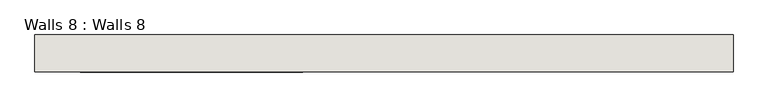
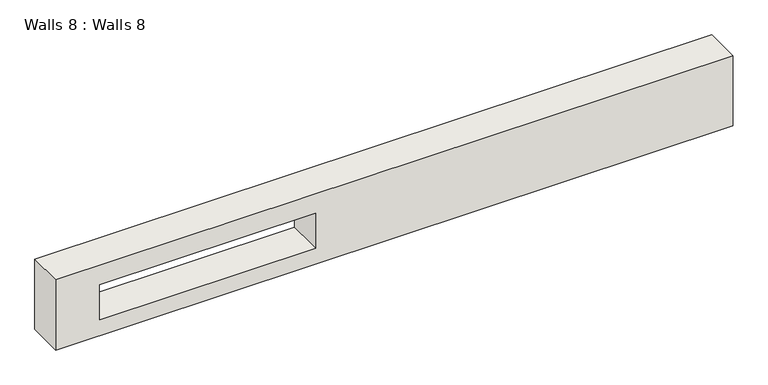
"""IFC4 building model written with IfcOpenShell, lengths in millimetres: wall geometry, Walls 8 : Walls 8."""

from ifc_helpers import new_model, si_unit, frame, origin, place, context, project, spatial, polyline, outline, extrude, source, transform, mapped, element, save


def walls_8_walls_8_f603c033(model_context):
    return source(origin(), model_context, "Body", "SweptSolid", [
        extrude(outline(polyline([(3969.8902454, 645.5980639), (3969.8902454, -5093.2019361), (3341.3717218, -5093.2019361), (3341.3717218, 645.5980639), (3969.8902454, 645.5980639)]), holes=[polyline([(3794.6218444, -2890.5343531), (3483.6009608, -2890.5343531), (3483.6009608, -4719.3343531), (3794.6218444, -4719.3343531), (3794.6218444, -2890.5343531)])]), frame((0.0, -6810.6562913, 0.0), z_axis=(0.0, 1.0, 0.0), x_axis=(0.0, 0.0, 1.0)), (0.0, 0.0, 1.0), 304.8),
    ])


if __name__ == "__main__":
    model = new_model("IFC4")
    model_context = context("Model", 3, world=origin())
    ifc_project = project(units=[si_unit("LENGTHUNIT", "METRE", prefix="MILLI")], contexts=[model_context])
    site = spatial("IfcSite", under=ifc_project)
    building = spatial("IfcBuilding", under=site)
    placement = place(None, origin())
    walls_8_walls_8_shape = walls_8_walls_8_f603c033(model_context)
    element("IfcWall", 1, ObjectType="Walls 8 : Walls 8", at=placement, inside=building, context=model_context, shape_type="MappedRepresentation", body=[
        mapped(walls_8_walls_8_shape, transform((0.0, 0.0, 0.0), x_axis=(1.0, 0.0, 0.0), y_axis=(0.0, 1.0, 0.0), z_axis=(0.0, 0.0, 1.0))),
    ])
    save(model, "model.ifc")

# Revit data of these elements
# Element 1 (IfcWall, "Walls 8 : Walls 8")
#   Materials on its faces: "Default Wall"
# Materials
#   "Default Wall": colour RGB 80 80 80, transparency 0
